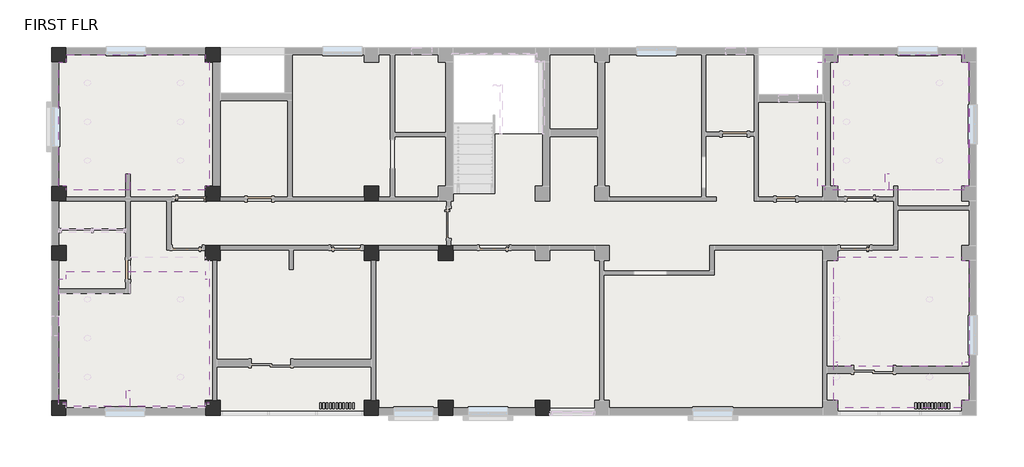
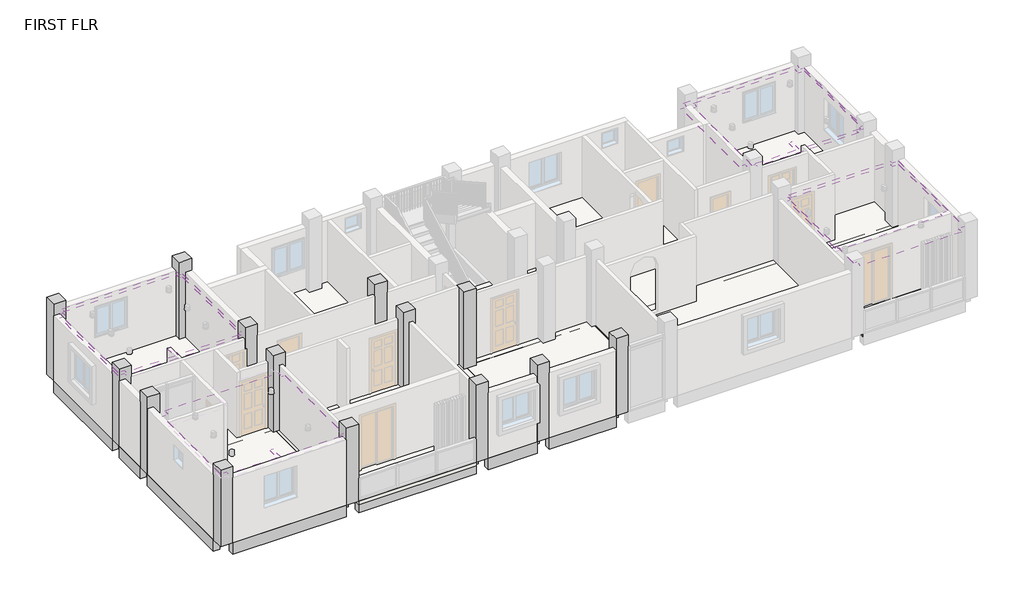
# One storey, part 3 of 5: 20 beams, 14 columns, 7 coverings, 3 slabs.
"""IFC4 building model written with IfcOpenShell, lengths in millimetres."""

from ifc_helpers import new_model, si_unit, point, frame, frame_2d, origin, place, context, project, spatial, polyline, circle_curve, trimmed, segment, composite_curve, outline, extrude, element, save

model = new_model("IFC4")

# Units and contexts
model_context = context("Model", 3, world=origin())
ifc_project = project(units=[si_unit("LENGTHUNIT", "METRE", prefix="MILLI")], contexts=[model_context])

# Site, building, storey
site = spatial("IfcSite", under=ifc_project)
building = spatial("IfcBuilding", under=site)
storey = spatial("IfcBuildingStorey", under=building, Name="FIRST FLR", Elevation=3352.8)

# Beams
placement = place(None, origin())
element("IfcBeam", 1, ObjectType="Concrete-Rectangular Beam : 9\" X 18\" BEAM", at=placement, inside=storey, context=model_context, shape_type="SweptSolid", body=[
    extrude(outline(polyline([(-10649.5456086, -10887.8679047), (-10649.5456086, -11116.4679047), (-14916.7456086, -11116.4679047), (-14916.7456086, -10887.8679047), (-10649.5456086, -10887.8679047)])), frame((0.0, 0.0, 2895.6), z_axis=(0.0, 0.0, 1.0), x_axis=(1.0, 0.0, 0.0)), (0.0, 0.0, 1.0), 457.2),
])
element("IfcBeam", 2, ObjectType="Concrete-Rectangular Beam : 9\" X 18\" BEAM", at=placement, inside=storey, context=model_context, shape_type="SweptSolid", body=[
    extrude(outline(polyline([(-5772.7456086, -10887.8679047), (-5772.7456086, -11116.4679047), (-10192.3456086, -11116.4679047), (-10192.3456086, -10887.8679047), (-5772.7456086, -10887.8679047)])), frame((0.0, 0.0, 2895.6), z_axis=(0.0, 0.0, 1.0), x_axis=(1.0, 0.0, 0.0)), (0.0, 0.0, 1.0), 457.2),
])
element("IfcBeam", 3, ObjectType="Concrete-Rectangular Beam : 9\" X 18\" BEAM", at=placement, inside=storey, context=model_context, shape_type="SweptSolid", body=[
    extrude(outline(polyline([(-3486.7456086, -10887.8679047), (-3486.7456086, -11116.4679047), (-5315.5456086, -11116.4679047), (-5315.5456086, -10887.8679047), (-3486.7456086, -10887.8679047)])), frame((0.0, 0.0, 2895.6), z_axis=(0.0, 0.0, 1.0), x_axis=(1.0, 0.0, 0.0)), (0.0, 0.0, 1.0), 457.2),
])
element("IfcBeam", 4, ObjectType="Concrete-Rectangular Beam : 9\" X 18\" BEAM", at=placement, inside=storey, context=model_context, shape_type="SweptSolid", body=[
    extrude(outline(polyline([(-518.4083398, -10887.8679047), (-518.4083398, -11116.4679047), (-3029.5456086, -11116.4679047), (-3029.5456086, -10887.8679047), (-518.4083398, -10887.8679047)])), frame((0.0, 0.0, 2895.6), z_axis=(0.0, 0.0, 1.0), x_axis=(1.0, 0.0, 0.0)), (0.0, 0.0, 1.0), 457.2),
])
element("IfcBeam", 5, ObjectType="Concrete-Rectangular Beam : 9\" X 18\" BEAM", at=placement, inside=storey, context=model_context, shape_type="SweptSolid", body=[
    extrude(outline(polyline([(-15145.3456086, -4072.3794704), (-15373.9456086, -4072.3794704), (-15373.9456086, -262.3794704), (-15145.3456086, -262.3794704), (-15145.3456086, -4072.3794704)])), frame((0.0, 0.0, 2895.6), z_axis=(0.0, 0.0, 1.0), x_axis=(1.0, 0.0, 0.0)), (0.0, 0.0, 1.0), 457.2),
])
element("IfcBeam", 6, ObjectType="Concrete-Rectangular Beam : 9\" X 18\" BEAM", at=placement, inside=storey, context=model_context, shape_type="SweptSolid", body=[
    extrude(outline(polyline([(-15145.3456086, -5901.1794704), (-15373.9456086, -5901.1794704), (-15373.9456086, -4529.5794704), (-15145.3456086, -4529.5794704), (-15145.3456086, -5901.1794704)])), frame((0.0, 0.0, 2895.6), z_axis=(0.0, 0.0, 1.0), x_axis=(1.0, 0.0, 0.0)), (0.0, 0.0, 1.0), 457.2),
])
element("IfcBeam", 7, ObjectType="Concrete-Rectangular Beam : 9\" X 18\" BEAM", at=placement, inside=storey, context=model_context, shape_type="SweptSolid", body=[
    extrude(outline(polyline([(-15145.3456086, -10659.2679047), (-15373.9456086, -10659.2679047), (-15373.9456086, -6358.3794704), (-15145.3456086, -6358.3794704), (-15145.3456086, -10659.2679047)])), frame((0.0, 0.0, 2895.6), z_axis=(0.0, 0.0, 1.0), x_axis=(1.0, 0.0, 0.0)), (0.0, 0.0, 1.0), 457.2),
])
element("IfcBeam", 8, ObjectType="Concrete-Rectangular Beam : 9\" X 18\" BEAM", at=placement, inside=storey, context=model_context, shape_type="SweptSolid", body=[
    extrude(outline(polyline([(-10649.5456086, -4186.6794704), (-10649.5456086, -4415.2794704), (-14916.7456086, -4415.2794704), (-14916.7456086, -4186.6794704), (-10649.5456086, -4186.6794704)])), frame((0.0, 0.0, 2895.6), z_axis=(0.0, 0.0, 1.0), x_axis=(1.0, 0.0, 0.0)), (0.0, 0.0, 1.0), 457.2),
])
element("IfcBeam", 9, ObjectType="Concrete-Rectangular Beam : 9\" X 18\" BEAM", at=placement, inside=storey, context=model_context, shape_type="SweptSolid", body=[
    extrude(outline(polyline([(-5772.7456086, -4186.6794704), (-5772.7456086, -4415.2794704), (-10192.3456086, -4415.2794704), (-10192.3456086, -4186.6794704), (-5772.7456086, -4186.6794704)])), frame((0.0, 0.0, 2895.6), z_axis=(0.0, 0.0, 1.0), x_axis=(1.0, 0.0, 0.0)), (0.0, 0.0, 1.0), 457.2),
])
element("IfcBeam", 10, ObjectType="Concrete-Rectangular Beam : 9\" X 18\" BEAM", at=placement, inside=storey, context=model_context, shape_type="SweptSolid", body=[
    extrude(outline(polyline([(-3486.7456086, -4186.6794704), (-3486.7456086, -4415.2794704), (-5315.5456086, -4415.2794704), (-5315.5456086, -4186.6794704), (-3486.7456086, -4186.6794704)])), frame((0.0, 0.0, 2895.6), z_axis=(0.0, 0.0, 1.0), x_axis=(1.0, 0.0, 0.0)), (0.0, 0.0, 1.0), 457.2),
])
element("IfcBeam", 11, ObjectType="Concrete-Rectangular Beam : 9\" X 18\" BEAM", at=placement, inside=storey, context=model_context, shape_type="SweptSolid", body=[
    extrude(outline(polyline([(-10306.6456086, -4072.3794704), (-10535.2456086, -4072.3794704), (-10535.2456086, -262.3794704), (-10306.6456086, -262.3794704), (-10306.6456086, -4072.3794704)])), frame((0.0, 0.0, 2895.6), z_axis=(0.0, 0.0, 1.0), x_axis=(1.0, 0.0, 0.0)), (0.0, 0.0, 1.0), 457.2),
])
element("IfcBeam", 12, ObjectType="Concrete-Rectangular Beam : 9\" X 18\" BEAM", at=placement, inside=storey, context=model_context, shape_type="SweptSolid", body=[
    extrude(outline(polyline([(-10649.5456086, -6015.4794704), (-10649.5456086, -6244.0794704), (-14916.7456086, -6244.0794704), (-14916.7456086, -6015.4794704), (-10649.5456086, -6015.4794704)])), frame((0.0, 0.0, 2895.6), z_axis=(0.0, 0.0, 1.0), x_axis=(1.0, 0.0, 0.0)), (0.0, 0.0, 1.0), 457.2),
])
element("IfcBeam", 13, ObjectType="Concrete-Rectangular Beam : 9\" X 18\" BEAM", at=placement, inside=storey, context=model_context, shape_type="SweptSolid", body=[
    extrude(outline(polyline([(-5772.7456086, -6015.4794704), (-5772.7456086, -6244.0794704), (-10192.3456086, -6244.0794704), (-10192.3456086, -6015.4794704), (-5772.7456086, -6015.4794704)])), frame((0.0, 0.0, 2895.6), z_axis=(0.0, 0.0, 1.0), x_axis=(1.0, 0.0, 0.0)), (0.0, 0.0, 1.0), 457.2),
])
element("IfcBeam", 14, ObjectType="Concrete-Rectangular Beam : 9\" X 18\" BEAM", at=placement, inside=storey, context=model_context, shape_type="SweptSolid", body=[
    extrude(outline(polyline([(-3486.7456086, -6015.4794704), (-3486.7456086, -6244.0794704), (-5315.5456086, -6244.0794704), (-5315.5456086, -6015.4794704), (-3486.7456086, -6015.4794704)])), frame((0.0, 0.0, 2895.6), z_axis=(0.0, 0.0, 1.0), x_axis=(1.0, 0.0, 0.0)), (0.0, 0.0, 1.0), 457.2),
])
element("IfcBeam", 15, ObjectType="Concrete-Rectangular Beam : 9\" X 18\" BEAM", at=placement, inside=storey, context=model_context, shape_type="SweptSolid", body=[
    extrude(outline(polyline([(-10535.2456086, -6358.3794704), (-10306.6456086, -6358.3794704), (-10306.6456086, -10659.2679047), (-10535.2456086, -10659.2679047), (-10535.2456086, -6358.3794704)])), frame((0.0, 0.0, 2895.6), z_axis=(0.0, 0.0, 1.0), x_axis=(1.0, 0.0, 0.0)), (0.0, 0.0, 1.0), 457.2),
])
element("IfcBeam", 16, ObjectType="Concrete-Rectangular Beam : 9\" X 18\" BEAM", at=placement, inside=storey, context=model_context, shape_type="SweptSolid", body=[
    extrude(outline(polyline([(-5658.4456086, -6358.3794704), (-5429.8456086, -6358.3794704), (-5429.8456086, -10659.2679047), (-5658.4456086, -10659.2679047), (-5658.4456086, -6358.3794704)])), frame((0.0, 0.0, 2895.6), z_axis=(0.0, 0.0, 1.0), x_axis=(1.0, 0.0, 0.0)), (0.0, 0.0, 1.0), 457.2),
])
element("IfcBeam", 17, ObjectType="Concrete-Rectangular Beam : 9\" X 18\" BEAM", at=placement, inside=storey, context=model_context, shape_type="SweptSolid", body=[
    extrude(outline(polyline([(-3372.4456086, -6358.3794704), (-3143.8456086, -6358.3794704), (-3143.8456086, -10659.2679047), (-3372.4456086, -10659.2679047), (-3372.4456086, -6358.3794704)])), frame((0.0, 0.0, 2895.6), z_axis=(0.0, 0.0, 1.0), x_axis=(1.0, 0.0, 0.0)), (0.0, 0.0, 1.0), 457.2),
])
element("IfcBeam", 18, ObjectType="Concrete-Rectangular Beam : 9\" X 18\" BEAM", at=placement, inside=storey, context=model_context, shape_type="SweptSolid", body=[
    extrude(outline(polyline([(-404.1083398, -6358.3794704), (-175.5083398, -6358.3794704), (-175.5083398, -10659.2679047), (-404.1083398, -10659.2679047), (-404.1083398, -6358.3794704)])), frame((0.0, 0.0, 2895.6), z_axis=(0.0, 0.0, 1.0), x_axis=(1.0, 0.0, 0.0)), (0.0, 0.0, 1.0), 457.2),
])
element("IfcBeam", 19, ObjectType="Concrete-Rectangular Beam : 9\" X 18\" BEAM", at=placement, inside=storey, context=model_context, shape_type="SweptSolid", body=[
    extrude(outline(polyline([(-5429.8456086, -5901.1794704), (-5658.4456086, -5901.1794704), (-5658.4456086, -4529.5794704), (-5429.8456086, -4529.5794704), (-5429.8456086, -5901.1794704)])), frame((0.0, 0.0, 2895.6), z_axis=(0.0, 0.0, 1.0), x_axis=(1.0, 0.0, 0.0)), (0.0, 0.0, 1.0), 457.2),
])
element("IfcBeam", 20, ObjectType="Concrete-Rectangular Beam : 9\" X 18\" BEAM", at=placement, inside=storey, context=model_context, shape_type="SweptSolid", body=[
    extrude(outline(polyline([(-10306.6456086, -5901.1794704), (-10535.2456086, -5901.1794704), (-10535.2456086, -4529.5794704), (-10306.6456086, -4529.5794704), (-10306.6456086, -5901.1794704)])), frame((0.0, 0.0, 2895.6), z_axis=(0.0, 0.0, 1.0), x_axis=(1.0, 0.0, 0.0)), (0.0, 0.0, 1.0), 457.2),
])

# Columns
element("IfcColumn", 21, ObjectType="Concrete-Rectangular-Column : COLUMN 18\" X 18\"", at=placement, inside=storey, context=model_context, shape_type="SweptSolid", body=[
    extrude(outline(polyline([(-14916.7456086, 194.8205296), (-14916.7456086, -262.3794704), (-15373.9456086, -262.3794704), (-15373.9456086, 194.8205296), (-14916.7456086, 194.8205296)])), frame((0.0, 0.0, 3352.8), z_axis=(0.0, 0.0, 1.0), x_axis=(1.0, 0.0, 0.0)), (0.0, 0.0, 1.0), 3048.0),
])
element("IfcColumn", 22, ObjectType="Concrete-Rectangular-Column : COLUMN 18\" X 18\"", at=placement, inside=storey, context=model_context, shape_type="SweptSolid", body=[
    extrude(outline(polyline([(-10192.3456086, 194.8205296), (-10192.3456086, -262.3794704), (-10649.5456086, -262.3794704), (-10649.5456086, 194.8205296), (-10192.3456086, 194.8205296)])), frame((0.0, 0.0, 3352.8), z_axis=(0.0, 0.0, 1.0), x_axis=(1.0, 0.0, 0.0)), (0.0, 0.0, 1.0), 3048.0),
])
element("IfcColumn", 23, ObjectType="Concrete-Rectangular-Column : COLUMN 18\" X 18\"", at=placement, inside=storey, context=model_context, shape_type="SweptSolid", body=[
    extrude(outline(polyline([(-61.2083398, -10659.2679047), (-61.2083398, -11116.4679047), (-518.4083398, -11116.4679047), (-518.4083398, -10659.2679047), (-61.2083398, -10659.2679047)])), frame((0.0, 0.0, 3352.8), z_axis=(0.0, 0.0, 1.0), x_axis=(1.0, 0.0, 0.0)), (0.0, 0.0, 1.0), 3048.0),
])
element("IfcColumn", 24, ObjectType="Concrete-Rectangular-Column : COLUMN 18\" X 18\"", at=placement, inside=storey, context=model_context, shape_type="SweptSolid", body=[
    extrude(outline(polyline([(-3029.5456086, -10659.2679047), (-3029.5456086, -11116.4679047), (-3486.7456086, -11116.4679047), (-3486.7456086, -10659.2679047), (-3029.5456086, -10659.2679047)])), frame((0.0, 0.0, 3352.8), z_axis=(0.0, 0.0, 1.0), x_axis=(1.0, 0.0, 0.0)), (0.0, 0.0, 1.0), 3048.0),
])
element("IfcColumn", 25, ObjectType="Concrete-Rectangular-Column : COLUMN 18\" X 18\"", at=placement, inside=storey, context=model_context, shape_type="SweptSolid", body=[
    extrude(outline(polyline([(-5315.5456086, -10659.2679047), (-5315.5456086, -11116.4679047), (-5772.7456086, -11116.4679047), (-5772.7456086, -10659.2679047), (-5315.5456086, -10659.2679047)])), frame((0.0, 0.0, 3352.8), z_axis=(0.0, 0.0, 1.0), x_axis=(1.0, 0.0, 0.0)), (0.0, 0.0, 1.0), 3048.0),
])
element("IfcColumn", 26, ObjectType="Concrete-Rectangular-Column : COLUMN 18\" X 18\"", at=placement, inside=storey, context=model_context, shape_type="SweptSolid", body=[
    extrude(outline(polyline([(-10192.3456086, -10659.2679047), (-10192.3456086, -11116.4679047), (-10649.5456086, -11116.4679047), (-10649.5456086, -10659.2679047), (-10192.3456086, -10659.2679047)])), frame((0.0, 0.0, 3352.8), z_axis=(0.0, 0.0, 1.0), x_axis=(1.0, 0.0, 0.0)), (0.0, 0.0, 1.0), 3048.0),
])
element("IfcColumn", 27, ObjectType="Concrete-Rectangular-Column : COLUMN 18\" X 18\"", at=placement, inside=storey, context=model_context, shape_type="SweptSolid", body=[
    extrude(outline(polyline([(-14916.7456086, -10659.2679047), (-14916.7456086, -11116.4679047), (-15373.9456086, -11116.4679047), (-15373.9456086, -10659.2679047), (-14916.7456086, -10659.2679047)])), frame((0.0, 0.0, 3352.8), z_axis=(0.0, 0.0, 1.0), x_axis=(1.0, 0.0, 0.0)), (0.0, 0.0, 1.0), 3048.0),
])
element("IfcColumn", 28, ObjectType="Concrete-Rectangular-Column : COLUMN 18\" X 18\"", at=placement, inside=storey, context=model_context, shape_type="SweptSolid", body=[
    extrude(outline(polyline([(-14916.7456086, -5901.1794704), (-14916.7456086, -6358.3794704), (-15373.9456086, -6358.3794704), (-15373.9456086, -5901.1794704), (-14916.7456086, -5901.1794704)])), frame((0.0, 0.0, 3352.8), z_axis=(0.0, 0.0, 1.0), x_axis=(1.0, 0.0, 0.0)), (0.0, 0.0, 1.0), 3048.0),
])
element("IfcColumn", 29, ObjectType="Concrete-Rectangular-Column : COLUMN 18\" X 18\"", at=placement, inside=storey, context=model_context, shape_type="SweptSolid", body=[
    extrude(outline(polyline([(-14916.7456086, -4072.3794704), (-14916.7456086, -4529.5794704), (-15373.9456086, -4529.5794704), (-15373.9456086, -4072.3794704), (-14916.7456086, -4072.3794704)])), frame((0.0, 0.0, 3352.8), z_axis=(0.0, 0.0, 1.0), x_axis=(1.0, 0.0, 0.0)), (0.0, 0.0, 1.0), 3048.0),
])
element("IfcColumn", 30, ObjectType="Concrete-Rectangular-Column : COLUMN 18\" X 18\"", at=placement, inside=storey, context=model_context, shape_type="SweptSolid", body=[
    extrude(outline(polyline([(-10192.3456086, -4072.3794704), (-10192.3456086, -4529.5794704), (-10649.5456086, -4529.5794704), (-10649.5456086, -4072.3794704), (-10192.3456086, -4072.3794704)])), frame((0.0, 0.0, 3352.8), z_axis=(0.0, 0.0, 1.0), x_axis=(1.0, 0.0, 0.0)), (0.0, 0.0, 1.0), 3048.0),
])
element("IfcColumn", 31, ObjectType="Concrete-Rectangular-Column : COLUMN 18\" X 18\"", at=placement, inside=storey, context=model_context, shape_type="SweptSolid", body=[
    extrude(outline(polyline([(-5315.5456086, -4072.3794704), (-5315.5456086, -4529.5794704), (-5772.7456086, -4529.5794704), (-5772.7456086, -4072.3794704), (-5315.5456086, -4072.3794704)])), frame((0.0, 0.0, 3352.8), z_axis=(0.0, 0.0, 1.0), x_axis=(1.0, 0.0, 0.0)), (0.0, 0.0, 1.0), 3048.0),
])
element("IfcColumn", 32, ObjectType="Concrete-Rectangular-Column : COLUMN 18\" X 18\"", at=placement, inside=storey, context=model_context, shape_type="SweptSolid", body=[
    extrude(outline(polyline([(-3029.5456086, -5901.1794704), (-3029.5456086, -6358.3794704), (-3486.7456086, -6358.3794704), (-3486.7456086, -5901.1794704), (-3029.5456086, -5901.1794704)])), frame((0.0, 0.0, 3352.8), z_axis=(0.0, 0.0, 1.0), x_axis=(1.0, 0.0, 0.0)), (0.0, 0.0, 1.0), 3048.0),
])
element("IfcColumn", 33, ObjectType="Concrete-Rectangular-Column : COLUMN 18\" X 18\"", at=placement, inside=storey, context=model_context, shape_type="SweptSolid", body=[
    extrude(outline(polyline([(-5315.5456086, -5901.1794704), (-5315.5456086, -6358.3794704), (-5772.7456086, -6358.3794704), (-5772.7456086, -5901.1794704), (-5315.5456086, -5901.1794704)])), frame((0.0, 0.0, 3352.8), z_axis=(0.0, 0.0, 1.0), x_axis=(1.0, 0.0, 0.0)), (0.0, 0.0, 1.0), 3048.0),
])
element("IfcColumn", 34, ObjectType="Concrete-Rectangular-Column : COLUMN 18\" X 18\"", at=placement, inside=storey, context=model_context, shape_type="SweptSolid", body=[
    extrude(outline(polyline([(-10192.3456086, -5901.1794704), (-10192.3456086, -6358.3794704), (-10649.5456086, -6358.3794704), (-10649.5456086, -5901.1794704), (-10192.3456086, -5901.1794704)])), frame((0.0, 0.0, 3352.8), z_axis=(0.0, 0.0, 1.0), x_axis=(1.0, 0.0, 0.0)), (0.0, 0.0, 1.0), 3048.0),
])

# Coverings
element("IfcCovering", 35, ObjectType="GWB on Mtl. Stud", at=placement, inside=storey, context=model_context, shape_type="SweptSolid", body=[
    extrude(outline(polyline([(-14916.7456086, -262.3794704), (-14916.7456086, -33.7794704), (-10649.5456086, -33.7794704), (-10649.5456086, -262.3794704), (-10535.2456086, -262.3794704), (-10535.2456086, -4072.3794704), (-10649.5456086, -4072.3794704), (-10649.5456086, -4186.6794704), (-12959.7401855, -4186.6794704), (-12959.7401855, -3705.5659448), (-13086.7401855, -3705.5659448), (-13086.7401855, -4186.6794704), (-14916.7456086, -4186.6794704), (-14916.7456086, -4072.3794704), (-15145.3456086, -4072.3794704), (-15145.3456086, -262.3794704), (-14916.7456086, -262.3794704)]), holes=[composite_curve([segment(trimmed(circle_curve(frame_2d((-14269.0456086, -897.3794704)), 76.2), [point((-14345.2456086, -897.3794704))], [point((-14192.8456086, -897.3794704))], True, "CARTESIAN"), True, "CONTINUOUS"), segment(trimmed(circle_curve(frame_2d((-14269.0456086, -897.3794704)), 76.2), [point((-14192.8456086, -897.3794704))], [point((-14345.2456086, -897.3794704))], True, "CARTESIAN"), True, "CONTINUOUS")], self_intersect=False), composite_curve([segment(trimmed(circle_curve(frame_2d((-14269.0456086, -3284.9794704)), 76.2), [point((-14345.2456086, -3284.9794704))], [point((-14192.8456086, -3284.9794704))], True, "CARTESIAN"), True, "CONTINUOUS"), segment(trimmed(circle_curve(frame_2d((-14269.0456086, -3284.9794704)), 76.2), [point((-14192.8456086, -3284.9794704))], [point((-14345.2456086, -3284.9794704))], True, "CARTESIAN"), True, "CONTINUOUS")], self_intersect=False), composite_curve([segment(trimmed(circle_curve(frame_2d((-14269.0456086, -2091.1794704)), 76.2), [point((-14345.2456086, -2091.1794704))], [point((-14192.8456086, -2091.1794704))], True, "CARTESIAN"), True, "CONTINUOUS"), segment(trimmed(circle_curve(frame_2d((-14269.0456086, -2091.1794704)), 76.2), [point((-14192.8456086, -2091.1794704))], [point((-14345.2456086, -2091.1794704))], True, "CARTESIAN"), True, "CONTINUOUS")], self_intersect=False), composite_curve([segment(trimmed(circle_curve(frame_2d((-11411.5456086, -897.3794704)), 76.2), [point((-11335.3456086, -897.3794704))], [point((-11487.7456086, -897.3794704))], True, "CARTESIAN"), True, "CONTINUOUS"), segment(trimmed(circle_curve(frame_2d((-11411.5456086, -897.3794704)), 76.2), [point((-11487.7456086, -897.3794704))], [point((-11335.3456086, -897.3794704))], True, "CARTESIAN"), True, "CONTINUOUS")], self_intersect=False), composite_curve([segment(trimmed(circle_curve(frame_2d((-11411.5456086, -3284.9794704)), 76.2), [point((-11335.3456086, -3284.9794704))], [point((-11487.7456086, -3284.9794704))], True, "CARTESIAN"), True, "CONTINUOUS"), segment(trimmed(circle_curve(frame_2d((-11411.5456086, -3284.9794704)), 76.2), [point((-11487.7456086, -3284.9794704))], [point((-11335.3456086, -3284.9794704))], True, "CARTESIAN"), True, "CONTINUOUS")], self_intersect=False), composite_curve([segment(trimmed(circle_curve(frame_2d((-11411.5456086, -2091.1794704)), 76.2), [point((-11335.3456086, -2091.1794704))], [point((-11487.7456086, -2091.1794704))], True, "CARTESIAN"), True, "CONTINUOUS"), segment(trimmed(circle_curve(frame_2d((-11411.5456086, -2091.1794704)), 76.2), [point((-11487.7456086, -2091.1794704))], [point((-11335.3456086, -2091.1794704))], True, "CARTESIAN"), True, "CONTINUOUS")], self_intersect=False)]), frame((0.0, 0.0, 5918.2), z_axis=(0.0, 0.0, 1.0), x_axis=(1.0, 0.0, 0.0)), (0.0, 0.0, 1.0), 107.95),
])
element("IfcCovering", 36, ObjectType="GWB on Mtl. Stud", at=placement, inside=storey, context=model_context, shape_type="SweptSolid", body=[
    extrude(outline(polyline([(-15145.3456086, -4072.3794704), (-15145.3456086, -262.3794704), (-14916.7456086, -262.3794704), (-14916.7456086, -33.7794704), (-10649.5456086, -33.7794704), (-10649.5456086, -262.3794704), (-10535.2456086, -262.3794704), (-10535.2456086, -4072.3794704), (-10649.5456086, -4072.3794704), (-10649.5456086, -4186.6794704), (-12959.7401855, -4186.6794704), (-14916.7456086, -4186.6794704), (-14916.7456086, -4072.3794704), (-15145.3456086, -4072.3794704)]), holes=[polyline([(-14840.5456086, -3881.8794704), (-10840.0456086, -3881.8794704), (-10840.0456086, -338.5794704), (-14840.5456086, -338.5794704), (-14840.5456086, -3881.8794704)])]), frame((0.0, 0.0, 5791.2), z_axis=(0.0, 0.0, 1.0), x_axis=(1.0, 0.0, 0.0)), (0.0, 0.0, 1.0), 107.95),
    extrude(outline(polyline([(-14688.1456086, -3729.4794704), (-14688.1456086, -490.9794704), (-10992.4456086, -490.9794704), (-10992.4456086, -3729.4794704), (-14688.1456086, -3729.4794704)]), holes=[polyline([(-11144.8456086, -643.3794704), (-14535.7456086, -643.3794704), (-14535.7456086, -3577.0794704), (-11144.8456086, -3577.0794704), (-11144.8456086, -643.3794704)])]), frame((0.0, 0.0, 5791.2), z_axis=(0.0, 0.0, 1.0), x_axis=(1.0, 0.0, 0.0)), (0.0, 0.0, 1.0), 107.95),
])
element("IfcCovering", 37, ObjectType="GWB on Mtl. Stud", at=placement, inside=storey, context=model_context, shape_type="SweptSolid", body=[
    extrude(outline(polyline([(8991.0043914, -3729.4794704), (8991.0043914, -490.9794704), (12477.1543914, -490.9794704), (12477.1543914, -3729.4794704), (8991.0043914, -3729.4794704)]), holes=[polyline([(12324.7543914, -643.3794704), (9162.4543914, -643.3794704), (9162.4543914, -3577.0794704), (12324.7543914, -3577.0794704), (12324.7543914, -643.3794704)])]), frame((0.0, 0.0, 5791.2), z_axis=(0.0, 0.0, 1.0), x_axis=(1.0, 0.0, 0.0)), (0.0, 0.0, 1.0), 107.95),
    extrude(outline(polyline([(8660.1098601, -4072.3794704), (8660.1098601, -262.3794704), (8774.4128058, -262.3794704), (8774.4128058, -33.7794704), (12584.4128058, -33.7794704), (12584.4128058, -262.3794704), (12813.0098601, -262.3794704), (12813.0098601, -4072.3794704), (12584.4128058, -4072.3794704), (12584.4128058, -4186.6794704), (10509.8598145, -4186.6794704), (8774.4128058, -4186.6794704), (8774.4128058, -4072.3794704), (8660.1098601, -4072.3794704)]), holes=[polyline([(8838.6043914, -338.5794704), (8838.6043914, -3881.8794704), (12629.5543914, -3881.8794704), (12629.5543914, -338.5794704), (8838.6043914, -338.5794704)])]), frame((0.0, 0.0, 5791.2), z_axis=(0.0, 0.0, 1.0), x_axis=(1.0, 0.0, 0.0)), (0.0, 0.0, 1.0), 107.95),
])
element("IfcCovering", 38, ObjectType="GWB on Mtl. Stud", at=placement, inside=storey, context=model_context, shape_type="SweptSolid", body=[
    extrude(outline(polyline([(8991.0043914, -9147.9642361), (8991.0043914, -6726.6794704), (12477.1543914, -6726.6794704), (12477.1543914, -9147.9642361), (8991.0043914, -9147.9642361)]), holes=[polyline([(12324.7543914, -7031.4298611), (9162.4543914, -7031.4298611), (9162.4543914, -8995.5642361), (12324.7543914, -8995.5642361), (12324.7543914, -7031.4298611)])]), frame((0.0, 0.0, 5791.2), z_axis=(0.0, 0.0, 1.0), x_axis=(1.0, 0.0, 0.0)), (0.0, 0.0, 1.0), 107.95),
    extrude(outline(polyline([(8660.1098601, -9490.8642361), (8660.1098601, -6358.3685356), (8774.4128058, -6358.3685356), (8774.4128058, -6244.0794704), (12584.4128058, -6244.0794704), (12584.4128058, -6358.3794704), (12813.0098601, -6358.3794704), (12813.0098601, -9490.8642361), (12584.4128058, -9490.8642361), (12584.4128058, -9605.1642361), (10509.8598145, -9605.1642361), (8774.4128058, -9605.1642361), (8774.4128058, -9490.8642361), (8660.1098601, -9490.8642361)]), holes=[polyline([(12629.5543914, -6498.0794704), (8838.6043914, -6498.0794704), (8838.6043914, -9300.3642361), (12629.5543914, -9300.3642361), (12629.5543914, -6498.0794704)])]), frame((0.0, 0.0, 5791.2), z_axis=(0.0, 0.0, 1.0), x_axis=(1.0, 0.0, 0.0)), (0.0, 0.0, 1.0), 107.95),
])
element("IfcCovering", 39, ObjectType="GWB on Mtl. Stud", at=placement, inside=storey, context=model_context, shape_type="SweptSolid", body=[
    extrude(outline(polyline([(8400.4543914, -262.3794704), (8400.4543914, -33.7794704), (12667.6543914, -33.7794704), (12667.6543914, -262.3794704), (12781.9543914, -262.3794704), (12781.9543914, -4072.3794704), (12667.6543914, -4072.3794704), (12667.6543914, -4186.6794704), (10357.4598145, -4186.6794704), (10357.4598145, -3705.5659448), (10230.4598145, -3705.5659448), (10230.4598145, -4186.6794704), (8400.4543914, -4186.6794704), (8400.4543914, -4072.3794704), (8171.8543914, -4072.3794704), (8171.8543914, -262.3794704), (8400.4543914, -262.3794704)]), holes=[composite_curve([segment(trimmed(circle_curve(frame_2d((9048.1543914, -897.3794704)), 76.2), [point((8971.9543914, -897.3794704))], [point((9124.3543914, -897.3794704))], True, "CARTESIAN"), True, "CONTINUOUS"), segment(trimmed(circle_curve(frame_2d((9048.1543914, -897.3794704)), 76.2), [point((9124.3543914, -897.3794704))], [point((8971.9543914, -897.3794704))], True, "CARTESIAN"), True, "CONTINUOUS")], self_intersect=False), composite_curve([segment(trimmed(circle_curve(frame_2d((9048.1543914, -3284.9794704)), 76.2), [point((8971.9543914, -3284.9794704))], [point((9124.3543914, -3284.9794704))], True, "CARTESIAN"), True, "CONTINUOUS"), segment(trimmed(circle_curve(frame_2d((9048.1543914, -3284.9794704)), 76.2), [point((9124.3543914, -3284.9794704))], [point((8971.9543914, -3284.9794704))], True, "CARTESIAN"), True, "CONTINUOUS")], self_intersect=False), composite_curve([segment(trimmed(circle_curve(frame_2d((9048.1543914, -2091.1794704)), 76.2), [point((8971.9543914, -2091.1794704))], [point((9124.3543914, -2091.1794704))], True, "CARTESIAN"), True, "CONTINUOUS"), segment(trimmed(circle_curve(frame_2d((9048.1543914, -2091.1794704)), 76.2), [point((9124.3543914, -2091.1794704))], [point((8971.9543914, -2091.1794704))], True, "CARTESIAN"), True, "CONTINUOUS")], self_intersect=False), composite_curve([segment(trimmed(circle_curve(frame_2d((11905.6543914, -897.3794704)), 76.2), [point((11981.8543914, -897.3794704))], [point((11829.4543914, -897.3794704))], True, "CARTESIAN"), True, "CONTINUOUS"), segment(trimmed(circle_curve(frame_2d((11905.6543914, -897.3794704)), 76.2), [point((11829.4543914, -897.3794704))], [point((11981.8543914, -897.3794704))], True, "CARTESIAN"), True, "CONTINUOUS")], self_intersect=False), composite_curve([segment(trimmed(circle_curve(frame_2d((11905.6543914, -3284.9794704)), 76.2), [point((11981.8543914, -3284.9794704))], [point((11829.4543914, -3284.9794704))], True, "CARTESIAN"), True, "CONTINUOUS"), segment(trimmed(circle_curve(frame_2d((11905.6543914, -3284.9794704)), 76.2), [point((11829.4543914, -3284.9794704))], [point((11981.8543914, -3284.9794704))], True, "CARTESIAN"), True, "CONTINUOUS")], self_intersect=False)]), frame((0.0, 0.0, 5918.2), z_axis=(0.0, 0.0, 1.0), x_axis=(1.0, 0.0, 0.0)), (0.0, 0.0, 1.0), 107.95),
])
element("IfcCovering", 40, ObjectType="GWB on Mtl. Stud", at=placement, inside=storey, context=model_context, shape_type="SweptSolid", body=[
    extrude(outline(polyline([(-14916.7456086, -6917.1794704), (-14916.7456086, -6688.5794704), (-10649.5456086, -6688.5794704), (-10649.5456086, -6917.1794704), (-10535.2456086, -6917.1794704), (-10535.2456086, -10727.1794704), (-10649.5456086, -10727.1794704), (-10649.5456086, -10841.4794704), (-12959.7401855, -10841.4794704), (-12959.7401855, -10360.3659448), (-13086.7401855, -10360.3659448), (-13086.7401855, -10841.4794704), (-14916.7456086, -10841.4794704), (-14916.7456086, -10727.1794704), (-15145.3456086, -10727.1794704), (-15145.3456086, -6917.1794704), (-14916.7456086, -6917.1794704)]), holes=[composite_curve([segment(trimmed(circle_curve(frame_2d((-14269.0456086, -7552.1794704)), 76.2), [point((-14345.2456086, -7552.1794704))], [point((-14192.8456086, -7552.1794704))], True, "CARTESIAN"), True, "CONTINUOUS"), segment(trimmed(circle_curve(frame_2d((-14269.0456086, -7552.1794704)), 76.2), [point((-14192.8456086, -7552.1794704))], [point((-14345.2456086, -7552.1794704))], True, "CARTESIAN"), True, "CONTINUOUS")], self_intersect=False), composite_curve([segment(trimmed(circle_curve(frame_2d((-14269.0456086, -9939.7794704)), 76.2), [point((-14345.2456086, -9939.7794704))], [point((-14192.8456086, -9939.7794704))], True, "CARTESIAN"), True, "CONTINUOUS"), segment(trimmed(circle_curve(frame_2d((-14269.0456086, -9939.7794704)), 76.2), [point((-14192.8456086, -9939.7794704))], [point((-14345.2456086, -9939.7794704))], True, "CARTESIAN"), True, "CONTINUOUS")], self_intersect=False), composite_curve([segment(trimmed(circle_curve(frame_2d((-14269.0456086, -8745.9794704)), 76.2), [point((-14345.2456086, -8745.9794704))], [point((-14192.8456086, -8745.9794704))], True, "CARTESIAN"), True, "CONTINUOUS"), segment(trimmed(circle_curve(frame_2d((-14269.0456086, -8745.9794704)), 76.2), [point((-14192.8456086, -8745.9794704))], [point((-14345.2456086, -8745.9794704))], True, "CARTESIAN"), True, "CONTINUOUS")], self_intersect=False), composite_curve([segment(trimmed(circle_curve(frame_2d((-11411.5456086, -7552.1794704)), 76.2), [point((-11335.3456086, -7552.1794704))], [point((-11487.7456086, -7552.1794704))], True, "CARTESIAN"), True, "CONTINUOUS"), segment(trimmed(circle_curve(frame_2d((-11411.5456086, -7552.1794704)), 76.2), [point((-11487.7456086, -7552.1794704))], [point((-11335.3456086, -7552.1794704))], True, "CARTESIAN"), True, "CONTINUOUS")], self_intersect=False), composite_curve([segment(trimmed(circle_curve(frame_2d((-11411.5456086, -9939.7794704)), 76.2), [point((-11335.3456086, -9939.7794704))], [point((-11487.7456086, -9939.7794704))], True, "CARTESIAN"), True, "CONTINUOUS"), segment(trimmed(circle_curve(frame_2d((-11411.5456086, -9939.7794704)), 76.2), [point((-11487.7456086, -9939.7794704))], [point((-11335.3456086, -9939.7794704))], True, "CARTESIAN"), True, "CONTINUOUS")], self_intersect=False)]), frame((0.0, 0.0, 5918.2), z_axis=(0.0, 0.0, 1.0), x_axis=(1.0, 0.0, 0.0)), (0.0, 0.0, 1.0), 107.95),
])
element("IfcCovering", 41, ObjectType="GWB on Mtl. Stud", at=placement, inside=storey, context=model_context, shape_type="SweptSolid", body=[
    extrude(outline(polyline([(8660.8043914, -6917.1794704), (8660.8043914, -6358.3794704), (8774.4128058, -6358.3794704), (8774.4128058, -6244.0794704), (12584.4128058, -6244.0794704), (12584.4128058, -6358.3794704), (12813.0098601, -6358.3794704), (12813.0098601, -10659.2679047), (12584.4128058, -10659.2679047), (12584.4128058, -10887.8673366), (8774.4128058, -10887.8673366), (8774.4128058, -10659.2679047), (8660.8043914, -10659.2679047), (8660.8043914, -6917.1794704)]), holes=[composite_curve([segment(trimmed(circle_curve(frame_2d((8743.3543914, -7552.1794704)), 76.2), [point((8667.1543914, -7552.1794704))], [point((8819.5543914, -7552.1794704))], True, "CARTESIAN"), True, "CONTINUOUS"), segment(trimmed(circle_curve(frame_2d((8743.3543914, -7552.1794704)), 76.2), [point((8819.5543914, -7552.1794704))], [point((8667.1543914, -7552.1794704))], True, "CARTESIAN"), True, "CONTINUOUS")], self_intersect=False), composite_curve([segment(trimmed(circle_curve(frame_2d((8743.3543914, -9939.7794704)), 76.2), [point((8667.1543914, -9939.7794704))], [point((8819.5543914, -9939.7794704))], True, "CARTESIAN"), True, "CONTINUOUS"), segment(trimmed(circle_curve(frame_2d((8743.3543914, -9939.7794704)), 76.2), [point((8819.5543914, -9939.7794704))], [point((8667.1543914, -9939.7794704))], True, "CARTESIAN"), True, "CONTINUOUS")], self_intersect=False), composite_curve([segment(trimmed(circle_curve(frame_2d((8743.3543914, -8745.9794704)), 76.2), [point((8667.1543914, -8745.9794704))], [point((8819.5543914, -8745.9794704))], True, "CARTESIAN"), True, "CONTINUOUS"), segment(trimmed(circle_curve(frame_2d((8743.3543914, -8745.9794704)), 76.2), [point((8819.5543914, -8745.9794704))], [point((8667.1543914, -8745.9794704))], True, "CARTESIAN"), True, "CONTINUOUS")], self_intersect=False), composite_curve([segment(trimmed(circle_curve(frame_2d((11600.8543914, -7552.1794704)), 76.2), [point((11677.0543914, -7552.1794704))], [point((11524.6543914, -7552.1794704))], True, "CARTESIAN"), True, "CONTINUOUS"), segment(trimmed(circle_curve(frame_2d((11600.8543914, -7552.1794704)), 76.2), [point((11524.6543914, -7552.1794704))], [point((11677.0543914, -7552.1794704))], True, "CARTESIAN"), True, "CONTINUOUS")], self_intersect=False), composite_curve([segment(trimmed(circle_curve(frame_2d((11600.8543914, -9939.7794704)), 76.2), [point((11677.0543914, -9939.7794704))], [point((11524.6543914, -9939.7794704))], True, "CARTESIAN"), True, "CONTINUOUS"), segment(trimmed(circle_curve(frame_2d((11600.8543914, -9939.7794704)), 76.2), [point((11524.6543914, -9939.7794704))], [point((11677.0543914, -9939.7794704))], True, "CARTESIAN"), True, "CONTINUOUS")], self_intersect=False)]), frame((0.0, 0.0, 5918.2), z_axis=(0.0, 0.0, 1.0), x_axis=(1.0, 0.0, 0.0)), (0.0, 0.0, 1.0), 107.95),
])

# Slabs
element("IfcSlab", 42, ObjectType="white MARBLE FLOORING 6\" 2", at=placement, inside=storey, context=model_context, shape_type="SweptSolid", body=[
    extrude(outline(polyline([(-14916.7456086, -262.3794704), (-14916.7456086, -33.7794704), (-10649.5456086, -33.7794704), (-10649.5456086, -262.3794704), (-10420.9456086, -262.3794704), (-10420.9456086, -4072.3794704), (-10649.5456086, -4072.3794704), (-10649.5456086, -4529.5794704), (-11614.7456086, -4529.5794704), (-11614.7456086, -4402.5794704), (-12959.7401855, -4402.5794704), (-12959.7401855, -3705.5659448), (-13086.7401855, -3705.5659448), (-13086.7401855, -4402.5794704), (-14916.7456086, -4402.5794704), (-14916.7456086, -4072.3794704), (-15145.3456086, -4072.3794704), (-15145.3456086, -262.3794704), (-14916.7456086, -262.3794704)])), frame((0.0, 0.0, 3200.4), z_axis=(0.0, 0.0, 1.0), x_axis=(1.0, 0.0, 0.0)), (0.0, 0.0, 1.0), 152.4),
    extrude(outline(polyline([(-15145.3456086, -7363.1659448), (-12959.7401855, -7363.1659448), (-12959.7401855, -4529.5794704), (-11829.4401855, -4529.5794704), (-11829.4401855, -6028.1794704), (-10649.5456086, -6028.1794704), (-10649.5456086, -6358.3794704), (-10420.9456086, -6358.3794704), (-10420.9456086, -10659.2679047), (-10649.5456086, -10659.2679047), (-10649.5456086, -10887.8679047), (-14916.7456086, -10887.8679047), (-14916.7456086, -10659.2679047), (-15145.3456086, -10659.2679047), (-15145.3456086, -7363.1659448)])), frame((0.0, 0.0, 3200.4), z_axis=(0.0, 0.0, 1.0), x_axis=(1.0, 0.0, 0.0)), (0.0, 0.0, 1.0), 152.4),
    extrude(outline(polyline([(-5772.7456086, -11116.4679047), (-10192.3456086, -11116.4679047), (-10192.3456086, -10659.2679047), (-10293.9456086, -10659.2679047), (-10293.9456086, -9630.5679047), (-9239.8456086, -9630.5679047), (-9239.8456086, -9401.9679047), (-10293.9456086, -9401.9679047), (-10293.9456086, -6358.3794704), (-10192.3456086, -6358.3794704), (-10192.3456086, -6028.1794704), (-8071.4456086, -6028.1794704), (-8071.4456086, -6637.7794704), (-7944.4456086, -6637.7794704), (-7944.4456086, -6028.1794704), (-6788.7456086, -6028.1794704), (-6788.7456086, -5901.1794704), (-5874.3456086, -5901.1794704), (-5874.3456086, -6028.1794704), (-5772.7456086, -6028.1794704), (-5772.7456086, -6358.3794704), (-5544.1456086, -6358.3794704), (-5544.1456086, -9401.9679047), (-8020.6456086, -9401.9679047), (-8020.6456086, -9630.5679047), (-5544.1456086, -9630.5679047), (-5544.1456086, -10659.2679047), (-5772.7456086, -10659.2679047), (-5772.7456086, -11116.4679047)])), frame((0.0, 0.0, 3200.4), z_axis=(0.0, 0.0, 1.0), x_axis=(1.0, 0.0, 0.0)), (0.0, 0.0, 1.0), 152.4),
    extrude(outline(polyline([(-5315.5456086, -10659.2679047), (-5417.1456086, -10659.2679047), (-5417.1456086, -6358.3794704), (-5315.5456086, -6358.3794704), (-5315.5456086, -6028.1794704), (-3486.7456086, -6028.1794704), (-3486.7456086, -6358.3794704), (-3029.5456086, -6358.3794704), (-3029.5456086, -6028.1794704), (-2231.1769742, -6028.1794704), (-2231.1769742, -5901.1794704), (-1316.7769742, -5901.1794704), (-1316.7769742, -6028.1794704), (-518.4083398, -6028.1794704), (-518.4083398, -6358.3794704), (-61.2083398, -6358.3794704), (-61.2083398, -6028.1794704), (1310.3916602, -6028.1794704), (1310.3916602, -6358.3794704), (1462.7916602, -6358.3794704), (1462.7916602, -10659.2679047), (1310.3916602, -10659.2679047), (1310.3916602, -10887.8679047), (-61.2083398, -10887.8679047), (-61.2083398, -10659.2679047), (-518.4083398, -10659.2679047), (-518.4083398, -10887.8679047), (-3029.5456086, -10887.8679047), (-3029.5456086, -10659.2679047), (-3486.7456086, -10659.2679047), (-3486.7456086, -10887.8679047), (-5315.5456086, -10887.8679047), (-5315.5456086, -10659.2679047)])), frame((0.0, 0.0, 3200.4), z_axis=(0.0, 0.0, 1.0), x_axis=(1.0, 0.0, 0.0)), (0.0, 0.0, 1.0), 152.4),
    extrude(outline(polyline([(1589.7916602, -6802.8794704), (4980.6916602, -6802.8794704), (4980.6916602, -6028.1794704), (8317.2128058, -6028.1794704), (8317.2128058, -10887.8679047), (1767.5916602, -10887.8679047), (1767.5916602, -10659.2679047), (1589.7916602, -10659.2679047), (1589.7916602, -6802.8794704)])), frame((0.0, 0.0, 3200.4), z_axis=(0.0, 0.0, 1.0), x_axis=(1.0, 0.0, 0.0)), (0.0, 0.0, 1.0), 152.4),
    extrude(outline(polyline([(8774.4128058, -10659.2679047), (8444.2128058, -10659.2679047), (8444.2128058, -9833.7679047), (9269.7128058, -9833.7679047), (9269.7128058, -9605.1679047), (8444.2128058, -9605.1679047), (8444.2128058, -6358.3794704), (8774.4128058, -6358.3794704), (8774.4128058, -6028.1794704), (8850.6128058, -6028.1794704), (8850.6128058, -5901.1794704), (9765.0128058, -5901.1794704), (9765.0128058, -6028.1794704), (9790.4128058, -6028.1794704), (10628.6128058, -6028.1794704), (10628.6128058, -4808.9794704), (12813.0128058, -4808.9794704), (12813.0128058, -5901.1794704), (12584.4128058, -5901.1794704), (12584.4128058, -6358.3794704), (12813.0128058, -6358.3794704), (12813.0128058, -9605.1679047), (10488.9128058, -9605.1679047), (10488.9128058, -9833.7679047), (12813.0128058, -9833.7679047), (12813.0128058, -10659.2679047), (12584.4128058, -10659.2679047), (12584.4128058, -11052.9679047), (8774.4128058, -11052.9679047), (8774.4128058, -10659.2679047)])), frame((0.0, 0.0, 3200.4), z_axis=(0.0, 0.0, 1.0), x_axis=(1.0, 0.0, 0.0)), (0.0, 0.0, 1.0), 152.4),
    extrude(outline(polyline([(9968.2128058, -4529.5794704), (9053.8128058, -4529.5794704), (8774.4128058, -4529.5794704), (8774.4128058, -4072.3794704), (8545.8128058, -4072.3794704), (8545.8128058, -262.3794704), (8774.4128058, -262.3794704), (8774.4128058, -33.7794704), (12584.4128058, -33.7794704), (12584.4128058, -262.3794704), (12813.0128058, -262.3794704), (12813.0128058, -4072.3794704), (12584.4128058, -4072.3794704), (12584.4128058, -4529.5794704), (12813.0128058, -4529.5794704), (12813.0128058, -4681.9794704), (10628.6128058, -4681.9794704), (10628.6128058, -4072.3794704), (10501.6128058, -4072.3794704), (10501.6128058, -4402.5794704), (9968.2128058, -4402.5794704), (9968.2128058, -4529.5794704)])), frame((0.0, 0.0, 3200.4), z_axis=(0.0, 0.0, 1.0), x_axis=(1.0, 0.0, 0.0)), (0.0, 0.0, 1.0), 152.4),
])
element("IfcSlab", 43, ObjectType="white MARBLE FLOORING 6\" 2", at=placement, inside=storey, context=model_context, shape_type="SweptSolid", body=[
    extrude(outline(polyline([(-11702.4401855, -5901.1794704), (-11702.4401855, -4529.5794704), (-8604.8456086, -4529.5794704), (-3232.7456086, -4529.5794704), (-3232.7456086, -4758.1794704), (-3105.7456086, -4758.1794704), (-3105.7456086, -4529.5794704), (-3029.5456086, -4529.5794704), (-3029.5456086, -4300.9794704), (-1759.5456086, -4300.9794704), (-1759.5456086, -2472.1794704), (-289.8083398, -2472.1794704), (-289.8083398, -4072.3794704), (-518.4083398, -4072.3794704), (-518.4083398, -4529.5794704), (-61.2083398, -4529.5794704), (-61.2083398, -2548.3794704), (1399.2916602, -2548.3794704), (1399.2916602, -4072.3794704), (1310.3916602, -4072.3794704), (1310.3916602, -4529.5794704), (5044.1916602, -4529.5794704), (5044.1916602, -4402.5794704), (4726.6916602, -4402.5794704), (4726.6916602, -2535.6794704), (6212.5916602, -2535.6794704), (6212.5916602, -4529.5794704), (10501.6128058, -4529.5794704), (10501.6128058, -5901.1794704), (4853.6916602, -5901.1794704), (4853.6916602, -6675.8794704), (1589.7916602, -6675.8794704), (1589.7916602, -6358.3794704), (1767.5916602, -6358.3794704), (1767.5916602, -5901.1794704), (-3105.7456086, -5901.1794704), (-3105.7456086, -5672.5794704), (-3232.7456086, -5672.5794704), (-3232.7456086, -5901.1794704), (-10750.542897, -5901.1794704), (-10750.542897, -6028.1794704), (-11664.942897, -6028.1794704), (-11664.942897, -5901.1794704), (-11702.4401855, -5901.1794704)])), frame((0.0, 0.0, 3200.4), z_axis=(0.0, 0.0, 1.0), x_axis=(1.0, 0.0, 0.0)), (0.0, 0.0, 1.0), 152.4),
])
element("IfcSlab", 44, ObjectType="white MARBLE FLOORING 6\" 2", at=placement, inside=storey, context=model_context, shape_type="SweptSolid", body=[
    extrude(outline(polyline([(-61.2083398, -2319.7794704), (-61.2083398, -33.7794704), (1310.3916602, -33.7794704), (1310.3916602, -262.3794704), (1399.2916602, -262.3794704), (1399.2916602, -2319.7794704), (-61.2083398, -2319.7794704)])), frame((0.0, 0.0, 3352.8), z_axis=(0.0, 0.0, 1.0), x_axis=(1.0, 0.0, 0.0)), (0.0, 0.0, 1.0), 152.4),
    extrude(outline(polyline([(1767.5916602, -4072.3794704), (1627.8916602, -4072.3794704), (1627.8916602, -262.3794704), (1767.5916602, -262.3794704), (1767.5916602, -33.7794704), (4599.6916602, -33.7794704), (4599.6916602, -4402.5794704), (1767.5916602, -4402.5794704), (1767.5916602, -4072.3794704)])), frame((0.0, 0.0, 3352.8), z_axis=(0.0, 0.0, 1.0), x_axis=(1.0, 0.0, 0.0)), (0.0, 0.0, 1.0), 152.4),
    extrude(outline(polyline([(6212.5916602, -33.7794704), (6212.5916602, -2408.6794704), (5996.6916602, -2408.6794704), (5996.6916602, -2535.6794704), (5234.6916602, -2535.6794704), (5234.6916602, -2408.6794704), (4726.6916602, -2408.6794704), (4726.6916602, -33.7794704), (6212.5916602, -33.7794704)])), frame((0.0, 0.0, 3352.8), z_axis=(0.0, 0.0, 1.0), x_axis=(1.0, 0.0, 0.0)), (0.0, 0.0, 1.0), 152.4),
    extrude(outline(polyline([(6885.6916602, -4402.5794704), (6339.5916602, -4402.5794704), (6339.5916602, -1481.5794704), (8418.8128058, -1481.5794704), (8418.8128058, -4072.3794704), (8317.2128058, -4072.3794704), (8317.2128058, -4402.5794704), (7495.2916602, -4402.5794704), (7495.2916602, -4529.5794704), (6885.6916602, -4529.5794704), (6885.6916602, -4402.5794704)])), frame((0.0, 0.0, 3352.8), z_axis=(0.0, 0.0, 1.0), x_axis=(1.0, 0.0, 0.0)), (0.0, 0.0, 1.0), 152.4),
    extrude(outline(polyline([(-3486.7456086, -4402.5794704), (-4832.9456086, -4402.5794704), (-4832.9456086, -2548.3794704), (-3258.1456086, -2548.3794704), (-3258.1456086, -4072.3794704), (-3486.7456086, -4072.3794704), (-3486.7456086, -4402.5794704)])), frame((0.0, 0.0, 3352.8), z_axis=(0.0, 0.0, 1.0), x_axis=(1.0, 0.0, 0.0)), (0.0, 0.0, 1.0), 152.4),
    extrude(outline(polyline([(-10192.3456086, -4402.5794704), (-10192.3456086, -1443.4794704), (-8109.5456086, -1443.4794704), (-8109.5456086, -4402.5794704), (-8604.8456086, -4402.5794704), (-8604.8456086, -4529.5794704), (-9366.8456086, -4529.5794704), (-9366.8456086, -4402.5794704), (-10192.3456086, -4402.5794704)])), frame((0.0, 0.0, 3352.8), z_axis=(0.0, 0.0, 1.0), x_axis=(1.0, 0.0, 0.0)), (0.0, 0.0, 1.0), 152.4),
    extrude(outline(polyline([(-4832.9456086, -2421.3794704), (-4832.9456086, -33.7794704), (-3486.7456086, -33.7794704), (-3486.7456086, -262.3794704), (-3258.1456086, -262.3794704), (-3258.1456086, -2421.3794704), (-4832.9456086, -2421.3794704)])), frame((0.0, 0.0, 3352.8), z_axis=(0.0, 0.0, 1.0), x_axis=(1.0, 0.0, 0.0)), (0.0, 0.0, 1.0), 152.4),
    extrude(outline(polyline([(-7982.5456086, -4402.5794704), (-7982.5456086, -33.7794704), (-5772.7456086, -33.7794704), (-5772.7456086, -262.3794704), (-5315.5456086, -262.3794704), (-5315.5456086, -33.7794704), (-4959.9456086, -33.7794704), (-4959.9456086, -4402.5794704), (-5315.5456086, -4402.5794704), (-5315.5456086, -4072.3794704), (-5772.7456086, -4072.3794704), (-5772.7456086, -4402.5794704), (-7982.5456086, -4402.5794704)])), frame((0.0, 0.0, 3352.8), z_axis=(0.0, 0.0, 1.0), x_axis=(1.0, 0.0, 0.0)), (0.0, 0.0, 1.0), 152.4),
    extrude(outline(polyline([(-15145.3456086, -5901.1794704), (-15145.3456086, -4529.5794704), (-13086.7401855, -4529.5794704), (-13086.7401855, -6334.4659448), (-12959.7401855, -6334.4659448), (-12959.7401855, -6944.0659448), (-13086.7401855, -6945.7574008), (-13086.7401855, -7236.1659448), (-15145.3456086, -7236.1659448), (-15145.3456086, -6358.3794704), (-14916.7456086, -6358.3794704), (-14916.7456086, -5901.1794704), (-15145.3456086, -5901.1794704)])), frame((0.0, 0.0, 3352.8), z_axis=(0.0, 0.0, 1.0), x_axis=(1.0, 0.0, 0.0)), (0.0, 0.0, 1.0), 152.4),
])

save(model, "model.ifc")

# Revit data of these elements
# Type "Concrete-Rectangular Beam : 9\" X 18\" BEAM"
#   Assembly Code = "B10"
#   Length [instance default] = 5' - 0"
#   b = 0' - 9"
#   h = 1' - 6"
#   Structural Material [instance default] = Concrete, Cast-in-Place gray
# Type "Concrete-Rectangular-Column : COLUMN 18\" X 18\""
#   Assembly Code = "B10"
#   b = 1' - 6"
#   h = 1' - 6"
#   Structural Material [instance default] = Concrete, Cast-in-Place gray
# Type "GWB on Mtl. Stud"
#   Assembly Code = "C3030220"
#   built-in parameter 1002203 = 1 (stored number, unit not read)
#   built-in parameter 1002202 = 1 (stored number, unit not read)
#   Layers, outside or top first: 0' - 3 5/8" "WHITE CEILING 6\"" (function 1); 0' - 0 5/8" "WHITE CEILING 6\"" (function 5)
# Type "white MARBLE FLOORING 6\" 2"
#   Assembly Code = "B1010"
#   Function = 0
#   Layers, outside or top first: 0' - 6" "MARBLE FLOORING 6\"" (function 1)
# Elements 1, 2, 3, 4, 5, 6, 7 (IfcBeam, "Concrete-Rectangular Beam : 9\" X 18\" BEAM")
#   Structural Material = Concrete, Cast-in-Place gray
#   Phase Created = New Construction
#   Materials on its faces: "Concrete, Cast-in-Place gray", "SAND BEIGE PAINT"
# Elements 8, 9, 10, 11, 12, 13, 14, 15, 16, 17, 18, 19, 20 (IfcBeam, "Concrete-Rectangular Beam : 9\" X 18\" BEAM")
#   Structural Material = Concrete, Cast-in-Place gray
#   Phase Created = New Construction
#   Materials on its faces: "Concrete, Cast-in-Place gray"
# Elements 21, 22, 23, 24, 25, 26, 27, 28, 29 (IfcColumn, "Concrete-Rectangular-Column : COLUMN 18\" X 18\"")
#   Structural Material = Concrete, Cast-in-Place gray
#   Phase Created = New Construction
#   Materials on its faces: "Concrete, Cast-in-Place gray", "SAND BEIGE PAINT"
# Elements 30, 31, 32, 33, 34 (IfcColumn, "Concrete-Rectangular-Column : COLUMN 18\" X 18\"")
#   Structural Material = Concrete, Cast-in-Place gray
#   Phase Created = New Construction
#   Materials on its faces: "Concrete, Cast-in-Place gray"
# Elements 35, 39, 40, 41 (IfcCovering, "GWB on Mtl. Stud")
#   Height Offset From Level = 8' - 5"
#   Phase Created = New Construction
#   Materials on its faces: "WHITE CEILING 6\""
# Elements 36, 37, 38 (IfcCovering, "GWB on Mtl. Stud")
#   Height Offset From Level = 8' - 0"
#   Phase Created = New Construction
#   Materials on its faces: "WHITE CEILING 6\""
# Element 42 (IfcSlab, "white MARBLE FLOORING 6\" 2")
#   Height Offset From Level = 0' - 0"
#   Phase Created = New Construction
#   Materials on its faces: "MARBLE FLOORING 6\""
# Element 43 (IfcSlab, "white MARBLE FLOORING 6\" 2")
#   built-in parameter 1001955 = -1.5708 (stored number, unit not read)
#   Height Offset From Level = 0' - 0"
#   Phase Created = New Construction
#   Materials on its faces: "MARBLE FLOORING 6\""
# Element 44 (IfcSlab, "white MARBLE FLOORING 6\" 2")
#   built-in parameter 1001955 = -1.5708 (stored number, unit not read)
#   Height Offset From Level = 0' - 6"
#   Phase Created = New Construction
#   Materials on its faces: "MARBLE FLOORING 6\""
# Materials
#   "Concrete, Cast-in-Place gray": class "Concrete", colour RGB 192 192 192, transparency 0, Description = "Cast-in-place concrete", Cost = 0
#   "WHITE CEILING 6\"": class "Generic", colour RGB 120 120 120, transparency 0, Cost = 0
#   "MARBLE FLOORING 6\"": class "Generic", colour RGB 120 120 120, transparency 0, Cost = 0
#   "SAND BEIGE PAINT": class "Generic", colour RGB 120 120 120, transparency 0, Cost = 0
